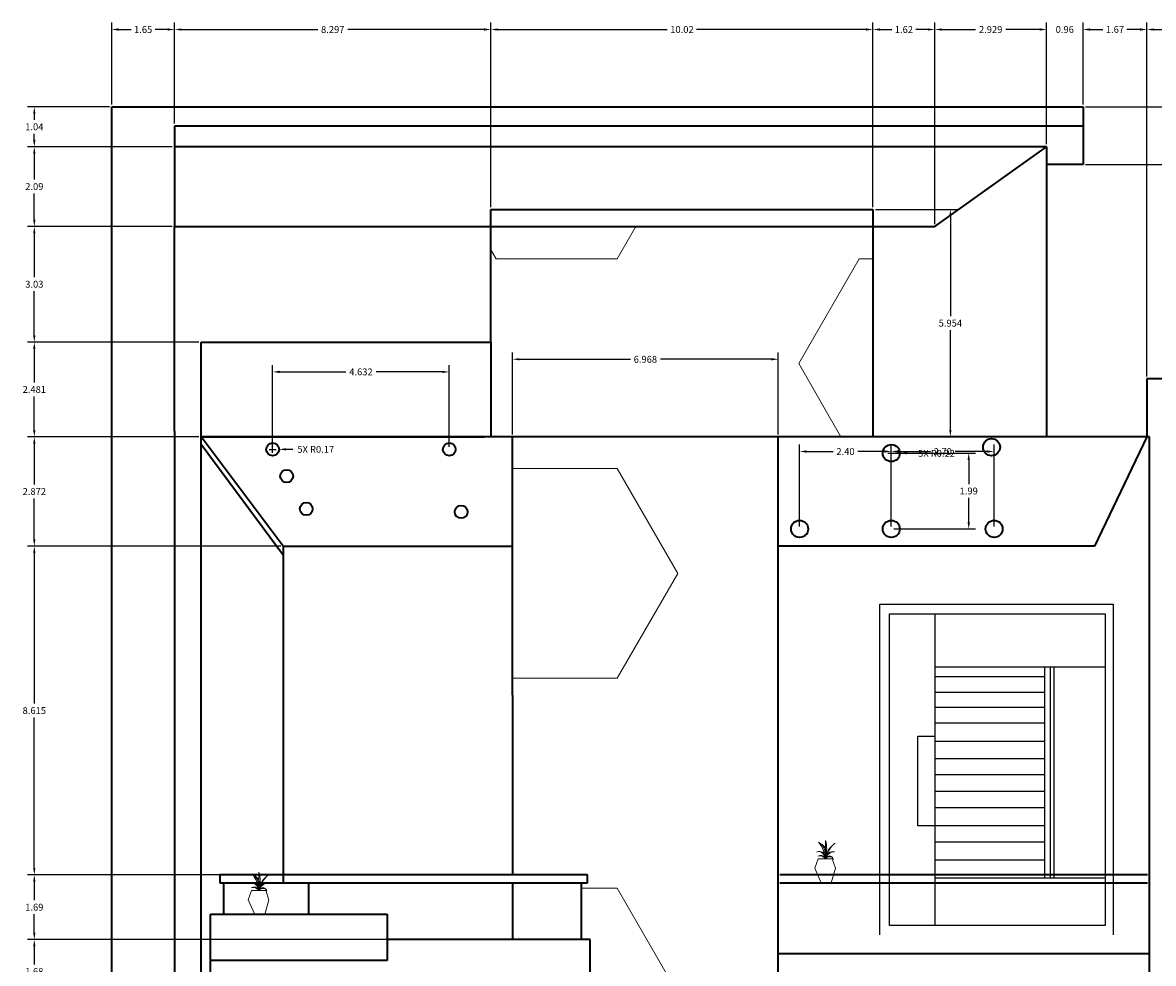
# Model space of a CAD drawing. Units: millimetres. Extents: x 2521.2 to 2565.9, y 755.2 to 798.1.
# Tile 2 of 3: x 2521.2 to 2550.9, y 773.4 to 798.1. Entities that reach past the tile are written whole.
import ezdxf

# ---------------------------------------------------------------- set-up
doc = ezdxf.new("R2010")
doc.units = ezdxf.units.MM
for name, color, linetype, lineweight in [('A-ANNO-DIMS', 2, 'Continuous', 18), ('A-DOOR', 3, 'Continuous', 25), ('A-ELEV', 7, 'Continuous', 35), ('A-WALL-PATT', 8, 'Continuous', 13), ('L-PLNT', 3, 'Continuous', 18)]:
    doc.layers.add(name, color=color, linetype=linetype, lineweight=lineweight)
doc.styles.get("Standard").update_dxf_attribs({"font": 'arial.ttf'})
doc.dimstyles.get("Standard").update_dxf_attribs({"dimtxt": 0.18, "dimasz": 0.18, "dimexe": 0.18, "dimexo": 0.0625, "dimgap": 0.09, "dimtad": 0, "dimtih": 1, "dimtoh": 1, "dimdec": 4, "dimzin": 0, "dimdsep": 46, "dimtxsty": 'Standard', "dimcen": 0.09, "dimadec": 0, "dimazin": 0, "dimtfac": 1, "dimtdec": 4, "dimtofl": 0, "dimtmove": 0, "dimatfit": 3, "dimfxl": 1, "dimtolj": 1, "dimtzin": 0, "dimarcsym": 0})

# ---------------------------------------------------------------- blocks, each defined once
blk = doc.blocks.new('DOOR-MAIN')
for p, q in [((2542.828, 758.373), (2542.828, 767.037)), ((2542.828, 767.037), (2548.944, 767.037)), ((2548.944, 767.037), (2548.944, 758.373)), ((2544.274, 766.783), (2544.274, 758.62)), ((2544.274, 765.396), (2548.734, 765.396)), ((2547.145, 765.396), (2547.145, 759.865)), ((2547.299, 765.396), (2547.299, 759.865)), ((2547.389, 765.396), (2547.389, 759.865)), ((2547.145, 765.132), (2544.274, 765.132)), ((2547.145, 764.725), (2544.274, 764.725)), ((2547.145, 764.331), (2544.274, 764.331)), ((2547.145, 763.924), (2544.274, 763.924)), ((2543.829, 761.227), (2543.829, 763.581)), ((2543.829, 763.581), (2544.274, 763.581)), ((2547.145, 763.441), (2544.274, 763.441)), ((2547.145, 762.983), (2544.274, 762.983)), ((2547.145, 762.564), (2544.274, 762.564)), ((2547.145, 762.131), (2544.274, 762.131)), ((2547.145, 761.699), (2544.274, 761.699)), ((2544.274, 761.227), (2543.829, 761.227)), ((2547.145, 761.227), (2544.274, 761.227)), ((2547.145, 760.804), (2544.274, 760.804)), ((2547.145, 760.33), (2544.274, 760.33)), ((2544.274, 759.865), (2548.734, 759.865))]:
    blk.add_line(p, q)
blk.add_lwpolyline([(2543.079, 766.783), (2548.734, 766.783), (2548.734, 758.62), (2543.079, 758.62)], close=True)
blk = doc.blocks.new('PLANTER')
for p, q in [((2558.646, 757.758), (2558.737, 758.005)), ((2558.817, 757.373), (2558.646, 757.758)), ((2558.737, 758.005), (2559.107, 758.005)), ((2559.08, 757.373), (2559.189, 757.758)), ((2559.189, 757.758), (2559.107, 758.005))]:
    blk.add_line(p, q)
for centre, radius, start, end in [((2558.504, 758.092), 0.427, 348.2161, 55.5831), ((2558.151, 757.944), 0.777, 5.6498, 40.0889), ((2558.161, 757.954), 0.763, 3.8104, 39.9888), ((2558.66, 758.146), 0.293, 333.1798, 63.2065), ((2558.164, 758.26), 0.796, 342.0282, 16.5628), ((2559.557, 757.89), 0.648, 126.493, 168.9551), ((2530.529, 758.527), 28.398, 358.9459, 359.9172), ((2559.736, 757.784), 0.843, 132.0051, 164.8224), ((2558.772, 758.043), 0.155, 345.7039, 120.8927), ((2558.788, 757.931), 0.154, 28.8769, 113.7957), ((2558.813, 757.985), 0.111, 10.1799, 119.9068), ((2558.697, 757.984), 0.226, 5.301, 71.0335), ((2559.127, 757.986), 0.208, 79.6534, 172.2119), ((2559.023, 757.968), 0.112, 7.4318, 155.8017), ((2559.176, 757.925), 0.266, 92.441, 162.4192), ((2559.033, 757.927), 0.136, 55.8779, 144.8755)]:
    blk.add_arc(centre, radius, start, end)
blk = doc.blocks.new('*D13')
at = {"layer": 'A-ANNO-DIMS', "color": 0, "lineweight": -2, "transparency": 16777216}
for p, q in [((2536.053, 774.051), (2521.361, 774.051)), ((2521.541, 773.871), (2521.541, 773.394)), ((2521.541, 772.553), (2521.541, 773.03)), ((2536.053, 772.373), (2521.361, 772.373))]:
    blk.add_line(p, q, dxfattribs=at)
at = {"layer": 'A-ANNO-DIMS', "color": 0, "transparency": 16777216}
for points in [[(2521.511, 773.871), (2521.571, 773.871), (2521.541, 774.051)], [(2521.511, 772.553), (2521.571, 772.553), (2521.541, 772.373)]]:
    blk.add_solid(points, dxfattribs=at)
at = {"layer": 'Defpoints', "color": 0, "transparency": 16777216}
for p in [(2521.541, 774.051), (2536.116, 774.051), (2536.116, 772.373)]:
    blk.add_point(p, dxfattribs=at)
at = {"layer": 'A-ANNO-DIMS', "color": 0, "transparency": 16777216, "insert": (2521.541, 773.212), "char_height": 0.18, "attachment_point": 5}
blk.add_mtext('\\A1;1.68', dxfattribs=at)
blk = doc.blocks.new('*D14')
at = {"layer": 'A-ANNO-DIMS', "color": 0, "lineweight": -2, "transparency": 16777216}
for p, q in [((2535.986, 775.744), (2521.361, 775.744)), ((2521.541, 775.564), (2521.541, 775.08)), ((2521.541, 774.231), (2521.541, 774.716)), ((2536.053, 774.051), (2521.361, 774.051))]:
    blk.add_line(p, q, dxfattribs=at)
at = {"layer": 'A-ANNO-DIMS', "color": 0, "transparency": 16777216}
for points in [[(2521.511, 775.564), (2521.571, 775.564), (2521.541, 775.744)], [(2521.511, 774.231), (2521.571, 774.231), (2521.541, 774.051)]]:
    blk.add_solid(points, dxfattribs=at)
at = {"layer": 'Defpoints', "color": 0, "transparency": 16777216}
for p in [(2521.541, 775.744), (2536.048, 775.744), (2536.116, 774.051)]:
    blk.add_point(p, dxfattribs=at)
at = {"layer": 'A-ANNO-DIMS', "color": 0, "transparency": 16777216, "insert": (2521.541, 774.898), "char_height": 0.18, "attachment_point": 5}
blk.add_mtext('\\A1;1.69', dxfattribs=at)
blk = doc.blocks.new('*D15')
at = {"layer": 'A-ANNO-DIMS', "color": 0, "lineweight": -2, "transparency": 16777216}
for p, q in [((2528.003, 784.359), (2521.361, 784.359)), ((2521.541, 784.179), (2521.541, 780.234)), ((2521.541, 775.924), (2521.541, 779.87)), ((2535.986, 775.744), (2521.361, 775.744))]:
    blk.add_line(p, q, dxfattribs=at)
at = {"layer": 'A-ANNO-DIMS', "color": 0, "transparency": 16777216}
for points in [[(2521.511, 784.179), (2521.571, 784.179), (2521.541, 784.359)], [(2521.511, 775.924), (2521.571, 775.924), (2521.541, 775.744)]]:
    blk.add_solid(points, dxfattribs=at)
at = {"layer": 'Defpoints', "color": 0, "transparency": 16777216}
for p in [(2521.541, 784.359), (2528.065, 784.359), (2536.048, 775.744)]:
    blk.add_point(p, dxfattribs=at)
at = {"layer": 'A-ANNO-DIMS', "color": 0, "transparency": 16777216, "insert": (2521.541, 780.052), "char_height": 0.18, "attachment_point": 5}
blk.add_mtext('\\A1;8.615', dxfattribs=at)
blk = doc.blocks.new('*D16')
at = {"layer": 'A-ANNO-DIMS', "color": 0, "lineweight": -2, "transparency": 16777216}
for p, q in [((2525.857, 787.231), (2521.361, 787.231)), ((2521.541, 787.051), (2521.541, 785.977)), ((2521.541, 784.539), (2521.541, 785.613)), ((2528.003, 784.359), (2521.361, 784.359))]:
    blk.add_line(p, q, dxfattribs=at)
at = {"layer": 'A-ANNO-DIMS', "color": 0, "transparency": 16777216}
for points in [[(2521.511, 787.051), (2521.571, 787.051), (2521.541, 787.231)], [(2521.511, 784.539), (2521.571, 784.539), (2521.541, 784.359)]]:
    blk.add_solid(points, dxfattribs=at)
at = {"layer": 'Defpoints', "color": 0, "transparency": 16777216}
for p in [(2521.541, 787.231), (2525.92, 787.231), (2528.065, 784.359)]:
    blk.add_point(p, dxfattribs=at)
at = {"layer": 'A-ANNO-DIMS', "color": 0, "transparency": 16777216, "insert": (2521.541, 785.795), "char_height": 0.18, "attachment_point": 5}
blk.add_mtext('\\A1;2.872', dxfattribs=at)
blk = doc.blocks.new('*D17')
at = {"layer": 'A-ANNO-DIMS', "color": 0, "lineweight": -2, "transparency": 16777216}
for p, q in [((2525.857, 789.712), (2521.361, 789.712)), ((2521.541, 789.532), (2521.541, 788.653)), ((2521.541, 787.411), (2521.541, 788.289)), ((2525.857, 787.231), (2521.361, 787.231))]:
    blk.add_line(p, q, dxfattribs=at)
at = {"layer": 'A-ANNO-DIMS', "color": 0, "transparency": 16777216}
for points in [[(2521.511, 789.532), (2521.571, 789.532), (2521.541, 789.712)], [(2521.511, 787.411), (2521.571, 787.411), (2521.541, 787.231)]]:
    blk.add_solid(points, dxfattribs=at)
at = {"layer": 'Defpoints', "color": 0, "transparency": 16777216}
for p in [(2521.541, 789.712), (2525.92, 789.712), (2525.92, 787.231)]:
    blk.add_point(p, dxfattribs=at)
at = {"layer": 'A-ANNO-DIMS', "color": 0, "transparency": 16777216, "insert": (2521.541, 788.471), "char_height": 0.18, "attachment_point": 5}
blk.add_mtext('\\A1;2.481', dxfattribs=at)
blk = doc.blocks.new('*D18')
at = {"layer": 'A-ANNO-DIMS', "color": 0, "lineweight": -2, "transparency": 16777216}
for p, q in [((2525.157, 792.744), (2521.361, 792.744)), ((2521.541, 792.564), (2521.541, 791.41)), ((2521.541, 789.892), (2521.541, 791.046)), ((2525.857, 789.712), (2521.361, 789.712))]:
    blk.add_line(p, q, dxfattribs=at)
at = {"layer": 'A-ANNO-DIMS', "color": 0, "transparency": 16777216}
for points in [[(2521.511, 792.564), (2521.571, 792.564), (2521.541, 792.744)], [(2521.511, 789.892), (2521.571, 789.892), (2521.541, 789.712)]]:
    blk.add_solid(points, dxfattribs=at)
at = {"layer": 'Defpoints', "color": 0, "transparency": 16777216}
for p in [(2521.541, 792.744), (2525.22, 792.744), (2525.92, 789.712)]:
    blk.add_point(p, dxfattribs=at)
at = {"layer": 'A-ANNO-DIMS', "color": 0, "transparency": 16777216, "insert": (2521.541, 791.228), "char_height": 0.18, "attachment_point": 5}
blk.add_mtext('\\A1;3.03', dxfattribs=at)
blk = doc.blocks.new('*D19')
at = {"layer": 'A-ANNO-DIMS', "color": 0, "lineweight": -2, "transparency": 16777216}
for p, q in [((2525.157, 794.834), (2521.361, 794.834)), ((2521.541, 794.654), (2521.541, 793.971)), ((2521.541, 792.924), (2521.541, 793.607)), ((2525.157, 792.744), (2521.361, 792.744))]:
    blk.add_line(p, q, dxfattribs=at)
at = {"layer": 'A-ANNO-DIMS', "color": 0, "transparency": 16777216}
for points in [[(2521.511, 794.654), (2521.571, 794.654), (2521.541, 794.834)], [(2521.511, 792.924), (2521.571, 792.924), (2521.541, 792.744)]]:
    blk.add_solid(points, dxfattribs=at)
at = {"layer": 'Defpoints', "color": 0, "transparency": 16777216}
for p in [(2521.541, 794.834), (2525.22, 794.834), (2525.22, 792.744)]:
    blk.add_point(p, dxfattribs=at)
at = {"layer": 'A-ANNO-DIMS', "color": 0, "transparency": 16777216, "insert": (2521.541, 793.789), "char_height": 0.18, "attachment_point": 5}
blk.add_mtext('\\A1;2.09', dxfattribs=at)
blk = doc.blocks.new('*D20')
at = {"layer": 'A-ANNO-DIMS', "color": 0, "lineweight": -2, "transparency": 16777216}
for p, q in [((2523.509, 795.876), (2521.361, 795.876)), ((2521.541, 795.696), (2521.541, 795.537)), ((2521.541, 795.014), (2521.541, 795.173)), ((2525.157, 794.834), (2521.361, 794.834))]:
    blk.add_line(p, q, dxfattribs=at)
at = {"layer": 'A-ANNO-DIMS', "color": 0, "transparency": 16777216}
for points in [[(2521.511, 795.696), (2521.571, 795.696), (2521.541, 795.876)], [(2521.511, 795.014), (2521.571, 795.014), (2521.541, 794.834)]]:
    blk.add_solid(points, dxfattribs=at)
at = {"layer": 'Defpoints', "color": 0, "transparency": 16777216}
for p in [(2521.541, 795.876), (2523.571, 795.876), (2525.22, 794.834)]:
    blk.add_point(p, dxfattribs=at)
at = {"layer": 'A-ANNO-DIMS', "color": 0, "transparency": 16777216, "insert": (2521.541, 795.355), "char_height": 0.18, "attachment_point": 5}
blk.add_mtext('\\A1;1.04', dxfattribs=at)
blk = doc.blocks.new('*D21')
at = {"layer": 'A-ANNO-DIMS', "color": 0, "lineweight": -2, "transparency": 16777216}
for p, q in [((2523.571, 795.939), (2523.571, 798.086)), ((2525.22, 795.439), (2525.22, 798.086)), ((2523.751, 797.906), (2524.079, 797.906)), ((2525.04, 797.906), (2524.711, 797.906))]:
    blk.add_line(p, q, dxfattribs=at)
at = {"layer": 'A-ANNO-DIMS', "color": 0, "transparency": 16777216}
for points in [[(2523.751, 797.936), (2523.751, 797.876), (2523.571, 797.906)], [(2525.04, 797.936), (2525.04, 797.876), (2525.22, 797.906)]]:
    blk.add_solid(points, dxfattribs=at)
at = {"layer": 'Defpoints', "color": 0, "transparency": 16777216}
for p in [(2525.22, 797.906), (2523.571, 795.876), (2525.22, 795.376)]:
    blk.add_point(p, dxfattribs=at)
at = {"layer": 'A-ANNO-DIMS', "color": 0, "transparency": 16777216, "insert": (2524.395, 797.906), "char_height": 0.18, "attachment_point": 5}
blk.add_mtext('\\A1;1.65', dxfattribs=at)
blk = doc.blocks.new('*D22')
at = {"layer": 'A-ANNO-DIMS', "color": 0, "lineweight": -2, "transparency": 16777216}
for p, q in [((2525.22, 795.439), (2525.22, 798.086)), ((2533.517, 793.248), (2533.517, 798.086)), ((2525.4, 797.906), (2528.974, 797.906)), ((2533.337, 797.906), (2529.762, 797.906))]:
    blk.add_line(p, q, dxfattribs=at)
at = {"layer": 'A-ANNO-DIMS', "color": 0, "transparency": 16777216}
for points in [[(2525.4, 797.936), (2525.4, 797.876), (2525.22, 797.906)], [(2533.337, 797.936), (2533.337, 797.876), (2533.517, 797.906)]]:
    blk.add_solid(points, dxfattribs=at)
at = {"layer": 'Defpoints', "color": 0, "transparency": 16777216}
for p in [(2533.517, 797.906), (2525.22, 795.376), (2533.517, 793.185)]:
    blk.add_point(p, dxfattribs=at)
at = {"layer": 'A-ANNO-DIMS', "color": 0, "transparency": 16777216, "insert": (2529.368, 797.906), "char_height": 0.18, "attachment_point": 5}
blk.add_mtext('\\A1;8.297', dxfattribs=at)
blk = doc.blocks.new('*D23')
at = {"layer": 'A-ANNO-DIMS', "color": 0, "lineweight": -2, "transparency": 16777216}
for p, q in [((2533.517, 793.248), (2533.517, 798.086)), ((2543.537, 793.248), (2543.537, 798.086)), ((2533.697, 797.906), (2538.142, 797.906)), ((2543.357, 797.906), (2538.911, 797.906))]:
    blk.add_line(p, q, dxfattribs=at)
at = {"layer": 'A-ANNO-DIMS', "color": 0, "transparency": 16777216}
for points in [[(2533.697, 797.936), (2533.697, 797.876), (2533.517, 797.906)], [(2543.357, 797.936), (2543.357, 797.876), (2543.537, 797.906)]]:
    blk.add_solid(points, dxfattribs=at)
at = {"layer": 'Defpoints', "color": 0, "transparency": 16777216}
for p in [(2543.537, 797.906), (2533.517, 793.185), (2543.537, 793.185)]:
    blk.add_point(p, dxfattribs=at)
at = {"layer": 'A-ANNO-DIMS', "color": 0, "transparency": 16777216, "insert": (2538.527, 797.906), "char_height": 0.18, "attachment_point": 5}
blk.add_mtext('\\A1;10.02', dxfattribs=at)
blk = doc.blocks.new('*D24')
at = {"layer": 'A-ANNO-DIMS', "color": 0, "lineweight": -2, "transparency": 16777216}
for p, q in [((2543.537, 793.248), (2543.537, 798.086)), ((2545.159, 792.807), (2545.159, 798.086)), ((2543.717, 797.906), (2544.034, 797.906)), ((2544.979, 797.906), (2544.662, 797.906))]:
    blk.add_line(p, q, dxfattribs=at)
at = {"layer": 'A-ANNO-DIMS', "color": 0, "transparency": 16777216}
for points in [[(2543.717, 797.936), (2543.717, 797.876), (2543.537, 797.906)], [(2544.979, 797.936), (2544.979, 797.876), (2545.159, 797.906)]]:
    blk.add_solid(points, dxfattribs=at)
at = {"layer": 'Defpoints', "color": 0, "transparency": 16777216}
for p in [(2545.159, 797.906), (2543.537, 793.185), (2545.159, 792.744)]:
    blk.add_point(p, dxfattribs=at)
at = {"layer": 'A-ANNO-DIMS', "color": 0, "transparency": 16777216, "insert": (2544.348, 797.906), "char_height": 0.18, "attachment_point": 5}
blk.add_mtext('\\A1;1.62', dxfattribs=at)
blk = doc.blocks.new('*D25')
at = {"layer": 'A-ANNO-DIMS', "color": 0, "lineweight": -2, "transparency": 16777216}
for p, q in [((2545.159, 792.807), (2545.159, 798.086)), ((2548.089, 794.896), (2548.089, 798.086)), ((2545.339, 797.906), (2546.228, 797.906)), ((2547.909, 797.906), (2547.019, 797.906))]:
    blk.add_line(p, q, dxfattribs=at)
at = {"layer": 'A-ANNO-DIMS', "color": 0, "transparency": 16777216}
for points in [[(2545.339, 797.936), (2545.339, 797.876), (2545.159, 797.906)], [(2547.909, 797.936), (2547.909, 797.876), (2548.089, 797.906)]]:
    blk.add_solid(points, dxfattribs=at)
at = {"layer": 'Defpoints', "color": 0, "transparency": 16777216}
for p in [(2548.089, 797.906), (2548.089, 794.834), (2545.159, 792.744)]:
    blk.add_point(p, dxfattribs=at)
at = {"layer": 'A-ANNO-DIMS', "color": 0, "transparency": 16777216, "insert": (2546.624, 797.906), "char_height": 0.18, "attachment_point": 5}
blk.add_mtext('\\A1;2.929', dxfattribs=at)
blk = doc.blocks.new('*D26')
at = {"layer": 'A-ANNO-DIMS', "color": 0, "lineweight": -2, "transparency": 16777216}
for p, q in [((2548.088503, 794.896188), (2548.088503, 798.086169)), ((2549.046391, 795.938669), (2549.046391, 798.086169)), ((2547.908503, 797.906169), (2547.728503, 797.906169)), ((2549.226391, 797.906169), (2549.406391, 797.906169))]:
    blk.add_line(p, q, dxfattribs=at)
at = {"layer": 'A-ANNO-DIMS', "color": 0, "transparency": 16777216}
for points in [[(2547.908503, 797.936169), (2547.908503, 797.876169), (2548.088503, 797.906169)], [(2549.226391, 797.936169), (2549.226391, 797.876169), (2549.046391, 797.906169)]]:
    blk.add_solid(points, dxfattribs=at)
at = {"layer": 'Defpoints', "color": 0, "transparency": 16777216}
for p in [(2549.046391, 797.906169), (2549.046391, 795.876169), (2548.088503, 794.833688)]:
    blk.add_point(p, dxfattribs=at)
at = {"layer": 'A-ANNO-DIMS', "color": 0, "transparency": 16777216, "insert": (2548.567447, 797.906169), "char_height": 0.18, "attachment_point": 5}
blk.add_mtext('\\A1;0.96', dxfattribs=at)
blk = doc.blocks.new('*D27')
at = {"layer": 'A-ANNO-DIMS', "color": 0, "lineweight": -2, "transparency": 16777216}
for p, q in [((2549.046, 795.939), (2549.046, 798.086)), ((2550.721, 788.812), (2550.721, 798.086)), ((2549.226, 797.906), (2549.568, 797.906)), ((2550.541, 797.906), (2550.199, 797.906))]:
    blk.add_line(p, q, dxfattribs=at)
at = {"layer": 'A-ANNO-DIMS', "color": 0, "transparency": 16777216}
for points in [[(2549.226, 797.936), (2549.226, 797.876), (2549.046, 797.906)], [(2550.541, 797.936), (2550.541, 797.876), (2550.721, 797.906)]]:
    blk.add_solid(points, dxfattribs=at)
at = {"layer": 'Defpoints', "color": 0, "transparency": 16777216}
for p in [(2550.721, 797.906), (2549.046, 795.876), (2550.721, 788.75)]:
    blk.add_point(p, dxfattribs=at)
at = {"layer": 'A-ANNO-DIMS', "color": 0, "transparency": 16777216, "insert": (2549.884, 797.906), "char_height": 0.18, "attachment_point": 5}
blk.add_mtext('\\A1;1.67', dxfattribs=at)
blk = doc.blocks.new('*D28')
at = {"layer": 'A-ANNO-DIMS', "color": 0, "lineweight": -2, "transparency": 16777216}
for p, q in [((2550.721, 788.812), (2550.721, 798.086)), ((2552.387, 788.812), (2552.387, 798.086)), ((2550.901, 797.906), (2551.169, 797.906)), ((2552.207, 797.906), (2551.939, 797.906))]:
    blk.add_line(p, q, dxfattribs=at)
at = {"layer": 'A-ANNO-DIMS', "color": 0, "transparency": 16777216}
for points in [[(2550.901, 797.936), (2550.901, 797.876), (2550.721, 797.906)], [(2552.207, 797.936), (2552.207, 797.876), (2552.387, 797.906)]]:
    blk.add_solid(points, dxfattribs=at)
at = {"layer": 'Defpoints', "color": 0, "transparency": 16777216}
for p in [(2552.387, 797.906), (2550.721, 788.75), (2552.387, 788.75)]:
    blk.add_point(p, dxfattribs=at)
at = {"layer": 'A-ANNO-DIMS', "color": 0, "transparency": 16777216, "insert": (2551.554, 797.906), "char_height": 0.18, "attachment_point": 5}
blk.add_mtext('\\A1;1.666', dxfattribs=at)
blk = doc.blocks.new('*D58')
at = {"layer": 'A-ANNO-DIMS', "color": 0, "lineweight": -2, "transparency": 16777216}
for p, q in [((2549.109, 794.365), (2565.781, 794.365)), ((2565.601, 794.185), (2565.601, 791.739)), ((2565.601, 788.93), (2565.601, 791.376)), ((2552.449, 788.75), (2565.781, 788.75))]:
    blk.add_line(p, q, dxfattribs=at)
at = {"layer": 'A-ANNO-DIMS', "color": 0, "transparency": 16777216}
for points in [[(2565.571, 794.185), (2565.631, 794.185), (2565.601, 794.365)], [(2565.571, 788.93), (2565.631, 788.93), (2565.601, 788.75)]]:
    blk.add_solid(points, dxfattribs=at)
at = {"layer": 'Defpoints', "color": 0, "transparency": 16777216}
for p in [(2549.046, 794.365), (2565.601, 794.365), (2552.387, 788.75)]:
    blk.add_point(p, dxfattribs=at)
at = {"layer": 'A-ANNO-DIMS', "color": 0, "transparency": 16777216, "insert": (2565.601, 791.557), "char_height": 0.18, "attachment_point": 5}
blk.add_mtext('\\A1;5.615', dxfattribs=at)
blk = doc.blocks.new('*D59')
at = {"layer": 'A-ANNO-DIMS', "color": 0, "lineweight": -2, "transparency": 16777216}
for p, q in [((2549.109, 795.876), (2565.781, 795.876)), ((2565.601, 795.696), (2565.601, 795.303)), ((2565.601, 794.545), (2565.601, 794.939)), ((2549.109, 794.365), (2565.781, 794.365))]:
    blk.add_line(p, q, dxfattribs=at)
at = {"layer": 'A-ANNO-DIMS', "color": 0, "transparency": 16777216}
for points in [[(2565.571, 795.696), (2565.631, 795.696), (2565.601, 795.876)], [(2565.571, 794.545), (2565.631, 794.545), (2565.601, 794.365)]]:
    blk.add_solid(points, dxfattribs=at)
at = {"layer": 'Defpoints', "color": 0, "transparency": 16777216}
for p in [(2549.046, 795.876), (2565.601, 795.876), (2549.046, 794.365)]:
    blk.add_point(p, dxfattribs=at)
at = {"layer": 'A-ANNO-DIMS', "color": 0, "transparency": 16777216, "insert": (2565.601, 795.121), "char_height": 0.18, "attachment_point": 5}
blk.add_mtext('\\A1;1.511', dxfattribs=at)
blk = doc.blocks.new('*D60')
at = {"layer": 'A-ANNO-DIMS', "color": 0, "lineweight": -2, "transparency": 16777216}
for p, q in [((2541.614, 784.875), (2541.614, 787.023)), ((2541.794, 786.843), (2542.491, 786.843)), ((2543.838, 786.843), (2543.141, 786.843)), ((2544.018, 784.875), (2544.018, 787.023))]:
    blk.add_line(p, q, dxfattribs=at)
at = {"layer": 'A-ANNO-DIMS', "color": 0, "transparency": 16777216}
for points in [[(2541.794, 786.873), (2541.794, 786.813), (2541.614, 786.843)], [(2543.838, 786.873), (2543.838, 786.813), (2544.018, 786.843)]]:
    blk.add_solid(points, dxfattribs=at)
at = {"layer": 'Defpoints', "color": 0, "transparency": 16777216}
for p in [(2544.018, 786.843), (2541.614, 784.813), (2544.018, 784.813)]:
    blk.add_point(p, dxfattribs=at)
at = {"layer": 'A-ANNO-DIMS', "color": 0, "transparency": 16777216, "insert": (2542.816, 786.843), "char_height": 0.18, "attachment_point": 5}
blk.add_mtext('\\A1;2.40', dxfattribs=at)
blk = doc.blocks.new('*D61')
at = {"layer": 'A-ANNO-DIMS', "color": 0, "lineweight": -2, "transparency": 16777216}
for p, q in [((2544.018, 784.875), (2544.018, 787.023)), ((2544.198, 786.843), (2545.042, 786.843)), ((2546.535, 786.843), (2545.692, 786.843)), ((2546.715, 784.875), (2546.715, 787.023))]:
    blk.add_line(p, q, dxfattribs=at)
at = {"layer": 'A-ANNO-DIMS', "color": 0, "transparency": 16777216}
for points in [[(2544.198, 786.873), (2544.198, 786.813), (2544.018, 786.843)], [(2546.535, 786.873), (2546.535, 786.813), (2546.715, 786.843)]]:
    blk.add_solid(points, dxfattribs=at)
at = {"layer": 'Defpoints', "color": 0, "transparency": 16777216}
for p in [(2546.715, 786.843), (2544.018, 784.813), (2546.715, 784.813)]:
    blk.add_point(p, dxfattribs=at)
at = {"layer": 'A-ANNO-DIMS', "color": 0, "transparency": 16777216, "insert": (2545.367, 786.843), "char_height": 0.18, "attachment_point": 5}
blk.add_mtext('\\A1;2.70', dxfattribs=at)
blk = doc.blocks.new('*D62')
at = {"layer": 'A-ANNO-DIMS', "color": 0, "lineweight": -2, "transparency": 16777216}
for p, q in [((2544.081, 786.802), (2546.228, 786.802)), ((2546.048, 786.622), (2546.048, 785.99)), ((2546.048, 784.993), (2546.048, 785.626)), ((2544.081, 784.813), (2546.228, 784.813))]:
    blk.add_line(p, q, dxfattribs=at)
at = {"layer": 'A-ANNO-DIMS', "color": 0, "transparency": 16777216}
for points in [[(2546.018, 786.622), (2546.078, 786.622), (2546.048, 786.802)], [(2546.018, 784.993), (2546.078, 784.993), (2546.048, 784.813)]]:
    blk.add_solid(points, dxfattribs=at)
at = {"layer": 'Defpoints', "color": 0, "transparency": 16777216}
for p in [(2544.018, 786.802), (2544.018, 784.813), (2546.048, 784.813)]:
    blk.add_point(p, dxfattribs=at)
at = {"layer": 'A-ANNO-DIMS', "color": 0, "transparency": 16777216, "insert": (2546.048, 785.808), "char_height": 0.18, "attachment_point": 5}
blk.add_mtext('\\A1;1.99', dxfattribs=at)
blk = doc.blocks.new('*D63')
at = {"layer": 'A-ANNO-DIMS', "color": 0, "lineweight": -2, "transparency": 16777216}
for p, q in [((2527.792, 786.962), (2527.792, 789.11)), ((2527.972, 788.93), (2529.712, 788.93)), ((2532.244, 788.93), (2530.504, 788.93)), ((2532.424, 786.962), (2532.424, 789.11))]:
    blk.add_line(p, q, dxfattribs=at)
at = {"layer": 'A-ANNO-DIMS', "color": 0, "transparency": 16777216}
for points in [[(2527.972, 788.96), (2527.972, 788.9), (2527.792, 788.93)], [(2532.244, 788.96), (2532.244, 788.9), (2532.424, 788.93)]]:
    blk.add_solid(points, dxfattribs=at)
at = {"layer": 'Defpoints', "color": 0, "transparency": 16777216}
for p in [(2532.424, 788.93), (2527.792, 786.9), (2532.424, 786.9)]:
    blk.add_point(p, dxfattribs=at)
at = {"layer": 'A-ANNO-DIMS', "color": 0, "transparency": 16777216, "insert": (2530.108, 788.93), "char_height": 0.18, "attachment_point": 5}
blk.add_mtext('\\A1;4.632', dxfattribs=at)
blk = doc.blocks.new('*D64')
at = {"layer": 'A-ANNO-DIMS', "color": 0, "lineweight": -2, "transparency": 16777216}
for p, q in [((2534.085, 787.293), (2534.085, 789.441)), ((2534.265, 789.261), (2537.174, 789.261)), ((2540.872, 789.261), (2537.963, 789.261)), ((2541.052, 787.293), (2541.052, 789.441))]:
    blk.add_line(p, q, dxfattribs=at)
at = {"layer": 'A-ANNO-DIMS', "color": 0, "transparency": 16777216}
for points in [[(2534.265, 789.291), (2534.265, 789.231), (2534.085, 789.261)], [(2540.872, 789.291), (2540.872, 789.231), (2541.052, 789.261)]]:
    blk.add_solid(points, dxfattribs=at)
at = {"layer": 'Defpoints', "color": 0, "transparency": 16777216}
for p in [(2541.052, 789.261), (2534.085, 787.231), (2541.052, 787.231)]:
    blk.add_point(p, dxfattribs=at)
at = {"layer": 'A-ANNO-DIMS', "color": 0, "transparency": 16777216, "insert": (2537.568, 789.261), "char_height": 0.18, "attachment_point": 5}
blk.add_mtext('\\A1;6.968', dxfattribs=at)
blk = doc.blocks.new('*D65')
at = {"layer": 'A-ANNO-DIMS', "color": 0, "lineweight": -2, "transparency": 16777216}
for p, q in [((2543.599, 793.185), (2545.747, 793.185)), ((2545.567, 793.005), (2545.567, 790.39)), ((2545.567, 787.411), (2545.567, 790.026)), ((2543.599, 787.231), (2545.747, 787.231))]:
    blk.add_line(p, q, dxfattribs=at)
at = {"layer": 'A-ANNO-DIMS', "color": 0, "transparency": 16777216}
for points in [[(2545.537, 793.005), (2545.597, 793.005), (2545.567, 793.185)], [(2545.537, 787.411), (2545.597, 787.411), (2545.567, 787.231)]]:
    blk.add_solid(points, dxfattribs=at)
at = {"layer": 'Defpoints', "color": 0, "transparency": 16777216}
for p in [(2543.537, 793.185), (2543.537, 787.231), (2545.567, 787.231)]:
    blk.add_point(p, dxfattribs=at)
at = {"layer": 'A-ANNO-DIMS', "color": 0, "transparency": 16777216, "insert": (2545.567, 790.208), "char_height": 0.18, "attachment_point": 5}
blk.add_mtext('\\A1;5.954', dxfattribs=at)
blk = doc.blocks.new('*D70')
at = {"layer": 'A-ANNO-DIMS', "color": 0, "lineweight": -2, "transparency": 16777216}
for p, q in [((2527.702, 786.9), (2527.882, 786.9)), ((2527.792, 786.81), (2527.792, 786.99)), ((2528.319, 786.9), (2528.139, 786.9))]:
    blk.add_line(p, q, dxfattribs=at)
at = {"layer": 'A-ANNO-DIMS', "color": 0, "transparency": 16777216}
blk.add_solid([(2528.139, 786.93), (2528.139, 786.87), (2527.959, 786.9)], dxfattribs=at)
at = {"layer": 'Defpoints', "color": 0, "transparency": 16777216}
for p in [(2527.792, 786.9), (2527.959, 786.9)]:
    blk.add_point(p, dxfattribs=at)
at = {"layer": 'A-ANNO-DIMS', "color": 0, "transparency": 16777216, "insert": (2528.923, 786.9), "char_height": 0.18, "attachment_point": 5}
blk.add_mtext('\\A1;5X R0.17', dxfattribs=at)
blk = doc.blocks.new('*D71')
at = {"layer": 'A-ANNO-DIMS', "color": 0, "lineweight": -2, "transparency": 16777216}
for p, q in [((2544.018, 786.712), (2544.018, 786.892)), ((2543.928, 786.802), (2544.108, 786.802)), ((2544.602, 786.795), (2544.422, 786.797))]:
    blk.add_line(p, q, dxfattribs=at)
at = {"layer": 'A-ANNO-DIMS', "color": 0, "transparency": 16777216}
blk.add_solid([(2544.422, 786.827), (2544.421, 786.767), (2544.242, 786.8)], dxfattribs=at)
at = {"layer": 'Defpoints', "color": 0, "transparency": 16777216}
for p in [(2544.018, 786.802), (2544.242, 786.8)]:
    blk.add_point(p, dxfattribs=at)
at = {"layer": 'A-ANNO-DIMS', "color": 0, "transparency": 16777216, "insert": (2545.204, 786.795), "char_height": 0.18, "attachment_point": 5}
blk.add_mtext('\\A1;5X R0.22', dxfattribs=at)

msp = doc.modelspace()

# ---------------------------------------------------------------- hatches: boundary and pattern name
at = {"layer": 'A-WALL-PATT'}
h = msp.add_hatch(dxfattribs=at)
h.set_pattern_fill('HEX', color=256)
h.paths.add_polyline_path([(2543.5368, 792.7443), (2533.5167, 792.7443), (2533.5167, 789.7118), (2533.5167, 787.2308), (2543.5368, 787.2308)])
h.paths.add_polyline_path([(2541.0523, 787.2308), (2534.0845, 787.2308), (2534.0845, 782.5843), (2534.0845, 780.4594), (2534.0845, 775.7444), (2536.0482, 775.7444), (2536.0482, 775.5347), (2535.8852, 775.5347), (2535.8852, 774.0509), (2536.1156, 774.0509), (2536.1156, 772.3734), (2535.8428, 772.3734), (2535.8428, 771.3734), (2541.0523, 771.3734), (2541.0523, 782.5843)])

# ---------------------------------------------------------------- linework, layer by layer
at = {"layer": 'A-ELEV'}
for p, q in [((2523.5711, 757.3734), (2523.5711, 795.8762)), ((2523.5711, 795.8762), (2549.0464, 795.8762)), ((2549.0464, 795.8762), (2549.0464, 795.376)), ((2549.0464, 795.376), (2525.2197, 795.376)), ((2525.2197, 795.376), (2525.2197, 794.8337)), ((2549.0464, 795.376), (2549.0464, 794.3652)), ((2548.0885, 794.8337), (2525.2197, 794.8337)), ((2525.2197, 794.8337), (2525.2197, 792.7443)), ((2545.1593, 792.7443), (2548.0885, 794.8337)), ((2548.0885, 794.8337), (2548.0885, 787.2308)), ((2549.0464, 794.3652), (2548.0885, 794.3652)), ((2533.5167, 792.7443), (2533.5167, 793.1853)), ((2533.5167, 793.1853), (2543.5368, 793.1853)), ((2543.5368, 793.1853), (2543.5368, 787.2308)), ((2525.2197, 787.3734), (2525.2197, 792.7443)), ((2525.2197, 792.7443), (2545.1593, 792.7443)), ((2533.5167, 789.7118), (2533.5167, 792.7443)), ((2525.9197, 787.2308), (2525.9197, 789.7118)), ((2525.9197, 789.7118), (2533.5167, 789.7118)), ((2533.5167, 789.7118), (2533.5167, 787.2308)), ((2552.1043, 788.7497), (2550.7207, 788.7497)), ((2550.7207, 788.7497), (2550.7207, 787.2308)), ((2525.2197, 787.3734), (2525.2197, 757.3734)), ((2525.9197, 757.3734), (2525.9197, 787.2308)), ((2525.9197, 787.2308), (2533.3485, 787.2308)), ((2550.7859, 787.2308), (2525.9197, 787.2308)), ((2528.0652, 784.3589), (2525.9197, 787.2308)), ((2534.0845, 782.5843), (2534.0845, 787.2308)), ((2541.0523, 782.5843), (2541.0523, 787.2308)), ((2550.7207, 787.2308), (2549.3434, 784.3589)), ((2550.7859, 782.5843), (2550.7859, 787.2308)), ((2528.0652, 784.1252), (2525.9197, 787.023)), ((2528.0652, 784.3589), (2534.0845, 784.3589)), ((2528.0652, 784.3589), (2528.0652, 775.5347)), ((2549.3434, 784.3589), (2541.0523, 784.3589)), ((2534.0845, 780.4594), (2534.0845, 782.5843)), ((2541.0523, 770.9792), (2541.0523, 782.5843)), ((2550.7859, 773.6725), (2550.7859, 782.5843)), ((2550.7859, 782.5843), (2550.7859, 782.5843)), ((2534.0845, 780.4594), (2534.0845, 775.7444)), ((2536.0482, 775.7444), (2526.408, 775.7444)), ((2526.408, 775.7444), (2526.408, 775.5347)), ((2536.0482, 775.5347), (2536.0482, 775.7444)), ((2550.7359, 775.7444), (2541.0957, 775.7444)), ((2526.408, 775.5347), (2536.0482, 775.5347)), ((2526.511, 774.7183), (2526.511, 775.5347)), ((2528.7319, 775.5347), (2528.7319, 774.7183)), ((2534.0845, 775.5347), (2534.0845, 774.0509)), ((2535.8852, 775.5347), (2535.8852, 774.0509)), ((2536.0482, 775.5347), (2536.0482, 775.5347)), ((2541.0957, 775.5347), (2550.7359, 775.5347)), ((2526.1636, 772.3734), (2526.1636, 774.7183)), ((2526.1636, 774.7183), (2530.7934, 774.7183)), ((2530.7934, 774.7183), (2530.7934, 773.5028)), ((2536.1156, 774.0509), (2530.7934, 774.0509)), ((2536.1156, 772.3734), (2536.1156, 774.0509)), ((2530.7934, 773.5028), (2526.1636, 773.5028)), ((2550.7859, 773.6725), (2541.0523, 773.6725)), ((2550.7859, 771.3734), (2550.7859, 773.6725))]:
    msp.add_line(p, q, dxfattribs=at)
for centre, radius in [((2546.6461, 786.9568), 0.2233), ((2527.7921, 786.8999), 0.1672), ((2532.4238, 786.8999), 0.1672), ((2544.0183, 786.8025), 0.2233), ((2528.1606, 786.1978), 0.1672), ((2528.6739, 785.3396), 0.1672), ((2532.7363, 785.2616), 0.1672), ((2541.6138, 784.8129), 0.2233), ((2544.0183, 784.8129), 0.2233), ((2546.7148, 784.8129), 0.2233)]:
    msp.add_circle(centre, radius, dxfattribs=at)

# ---------------------------------------------------------------- block references
at = {"layer": 'A-DOOR'}
msp.add_blockref('DOOR-MAIN', (0.8886, 15.8014), dxfattribs=at)
at = {"layer": 'L-PLNT'}
for p in [(-16.6359, 18.1614), (-31.4957, 17.3314)]:
    msp.add_blockref('PLANTER', p, dxfattribs=at)

# ---------------------------------------------------------------- dimensions: what is measured, and where the dimension line sits
at = {"layer": 'A-ANNO-DIMS'}
for base, p1, p2, override, picture, middle in [((2525.2197, 797.9062), (2523.5711, 795.8762), (2525.2197, 795.376), {"dimdec": 2, "dimlfac": 1, "dimrnd": 0, "dimzin": 0, "dimdsep": 46, "dimlunit": 2}, '*D21', (2524.3954, 797.9062)), ((2533.5167, 797.9062), (2525.2197, 795.376), (2533.5167, 793.1853), {"dimdec": 3, "dimlfac": 1, "dimrnd": 0, "dimzin": 0, "dimdsep": 46, "dimlunit": 2}, '*D22', (2529.3682, 797.9062)), ((2543.5368, 797.9062), (2533.5167, 793.1853), (2543.5368, 793.1853), {"dimdec": 2, "dimlfac": 1, "dimrnd": 0, "dimzin": 0, "dimdsep": 46, "dimlunit": 2}, '*D23', (2538.5268, 797.9062)), ((2545.1593, 797.9062), (2543.5368, 793.1853), (2545.1593, 792.7443), {"dimdec": 2, "dimlfac": 1, "dimrnd": 0, "dimzin": 0, "dimdsep": 46, "dimlunit": 2}, '*D24', (2544.3481, 797.9062)), ((2548.0885, 797.9062), (2545.1593, 792.7443), (2548.0885, 794.8337), {"dimdec": 3, "dimlfac": 1, "dimrnd": 0, "dimzin": 0, "dimdsep": 46, "dimlunit": 2}, '*D25', (2546.6239, 797.9062)), ((2549.0464, 797.9062), (2548.0885, 794.8337), (2549.0464, 795.8762), {"dimdec": 2, "dimlfac": 1, "dimrnd": 0, "dimzin": 0, "dimdsep": 46, "dimlunit": 2}, '*D26', (2548.5674, 797.9062)), ((2550.7207, 797.9062), (2549.0464, 795.8762), (2550.7207, 788.7497), {"dimdec": 2, "dimlfac": 1, "dimrnd": 0, "dimzin": 0, "dimdsep": 46, "dimlunit": 2}, '*D27', (2549.8835, 797.9062)), ((2552.3868, 797.9062), (2550.7207, 788.7497), (2552.3868, 788.7497), {"dimdec": 3, "dimlfac": 1, "dimrnd": 0, "dimzin": 0, "dimdsep": 46, "dimlunit": 2}, '*D28', (2551.5538, 797.9062)), ((2541.0523, 789.2608), (2534.0845, 787.2308), (2541.0523, 787.2308), {"dimdec": 3, "dimlfac": 1, "dimrnd": 0, "dimzin": 0, "dimdsep": 46, "dimlunit": 2}, '*D64', (2537.5684, 789.2608)), ((2532.4238, 788.9299), (2527.7921, 786.8999), (2532.4238, 786.8999), {"dimdec": 3, "dimlfac": 1, "dimrnd": 0, "dimzin": 0, "dimdsep": 46, "dimlunit": 2}, '*D63', (2530.1079, 788.9299)), ((2546.7148, 786.8429), (2544.0183, 784.8129), (2546.7148, 784.8129), {"dimdec": 2, "dimlfac": 1, "dimrnd": 0, "dimzin": 0, "dimdsep": 46, "dimlunit": 2}, '*D61', (2545.3665, 786.8429))]:
    dim = msp.add_linear_dim(base=base, p1=p1, p2=p2, dimstyle='Standard', override=override, dxfattribs=at)
    dim.commit()
    dim.dimension.update_dxf_attribs({"geometry": picture, "text_midpoint": middle})
for base, p1, p2, angle, override, picture, middle in [((2521.5411, 795.8762), (2525.2197, 794.8337), (2523.5711, 795.8762), 90, {"dimdec": 2, "dimlfac": 1, "dimrnd": 0, "dimzin": 0, "dimdsep": 46, "dimlunit": 2}, '*D20', (2521.5411, 795.3549)), ((2565.6011, 795.8762), (2549.0464, 794.3652), (2549.0464, 795.8762), 90, {"dimdec": 3, "dimlfac": 1, "dimrnd": 0, "dimzin": 0, "dimdsep": 46, "dimlunit": 2}, '*D59', (2565.6011, 795.1207)), ((2521.5411, 794.8337), (2525.2197, 792.7443), (2525.2197, 794.8337), 90, {"dimdec": 2, "dimlfac": 1, "dimrnd": 0, "dimzin": 0, "dimdsep": 46, "dimlunit": 2}, '*D19', (2521.5411, 793.789)), ((2565.60106, 794.36515), (2552.38684, 788.7497), (2549.04639, 794.36515), 90, {"dimdec": 3, "dimlfac": 1, "dimrnd": 0, "dimzin": 0, "dimdsep": 46, "dimlunit": 2}, '*D58', (2565.60106, 791.55743)), ((2545.56685, 787.23079), (2543.53685, 793.18528), (2543.53685, 787.23079), 270, {"dimdec": 3, "dimlfac": 1, "dimrnd": 0, "dimzin": 0, "dimdsep": 46, "dimlunit": 2}, '*D65', (2545.56685, 790.20803)), ((2521.5411, 792.7443), (2525.9197, 789.7118), (2525.2197, 792.7443), 90, {"dimdec": 2, "dimlfac": 1, "dimrnd": 0, "dimzin": 0, "dimdsep": 46, "dimlunit": 2}, '*D18', (2521.5411, 791.228)), ((2521.5411, 789.7118), (2525.9197, 787.2308), (2525.9197, 789.7118), 90, {"dimdec": 3, "dimlfac": 1, "dimrnd": 0, "dimzin": 0, "dimdsep": 46, "dimlunit": 2}, '*D17', (2521.5411, 788.4713)), ((2521.5411, 787.2308), (2528.0652, 784.3589), (2525.9197, 787.2308), 90, {"dimdec": 3, "dimlfac": 1, "dimrnd": 0, "dimzin": 0, "dimdsep": 46, "dimlunit": 2}, '*D16', (2521.5411, 785.7949)), ((2544.0183, 786.8429), (2541.6138, 784.8129), (2544.0183, 784.8129), 0, {"dimdec": 2, "dimlfac": 1, "dimrnd": 0, "dimzin": 0, "dimdsep": 46, "dimlunit": 2}, '*D60', (2542.816, 786.8429)), ((2546.0483, 784.8129), (2544.0183, 786.8025), (2544.0183, 784.8129), 270, {"dimdec": 2, "dimlfac": 1, "dimrnd": 0, "dimzin": 0, "dimdsep": 46, "dimlunit": 2}, '*D62', (2546.0483, 785.8077)), ((2521.54106, 784.35895), (2536.04816, 775.74436), (2528.06525, 784.35895), 90, {"dimdec": 3, "dimlfac": 1, "dimrnd": 0, "dimzin": 0, "dimdsep": 46, "dimlunit": 2}, '*D15', (2521.54106, 780.05165)), ((2521.5411, 775.7444), (2536.1156, 774.0509), (2536.0482, 775.7444), 90, {"dimdec": 2, "dimlfac": 1, "dimrnd": 0, "dimzin": 0, "dimdsep": 46, "dimlunit": 2}, '*D14', (2521.5411, 774.8977)), ((2521.5411, 774.0509), (2536.1156, 772.3734), (2536.1156, 774.0509), 90, {"dimdec": 2, "dimlfac": 1, "dimrnd": 0, "dimzin": 0, "dimdsep": 46, "dimlunit": 2}, '*D13', (2521.5411, 773.2122))]:
    dim = msp.add_linear_dim(base=base, p1=p1, p2=p2, angle=angle, dimstyle='Standard', override=override, dxfattribs=at)
    dim.commit()
    dim.dimension.update_dxf_attribs({"geometry": picture, "text_midpoint": middle})
for center, mpoint, picture, middle in [((2527.7921, 786.8999), (2527.9592, 786.9), '*D70', (2528.9225, 786.9002)), ((2544.0183, 786.8025), (2544.2415, 786.7996), '*D71', (2545.2039, 786.7949))]:
    dim = msp.add_radius_dim(center=center, mpoint=mpoint, text='5X <>', dimstyle='Standard', override={"dimdec": 2, "dimlfac": 1, "dimrnd": 0, "dimzin": 0, "dimdsep": 46, "dimlunit": 2}, dxfattribs=at)
    dim.commit()
    dim.dimension.update_dxf_attribs({"geometry": picture, "text_midpoint": middle})

doc.saveas('drawing.dxf')
